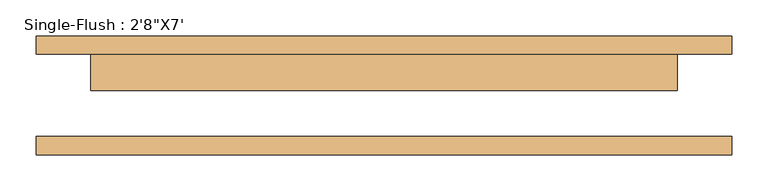
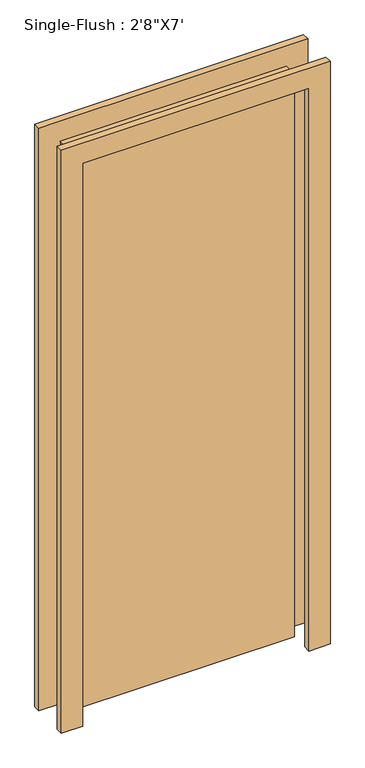
"""IFC4 building model written with IfcOpenShell, lengths in millimetres: door geometry."""

from ifc_helpers import new_model, si_unit, frame, origin, origin_with_axes, place, context, project, spatial, polyline, outline, extrude, source, transform, mapped, element, save


def door_d141acb4(model_context):
    return source(origin(), model_context, "Body", "SweptSolid", [
        extrude(outline(polyline([(2209.8, -482.6), (0.0, -482.6), (0.0, -406.4), (2133.6, -406.4), (2133.6, 406.4), (0.0, 406.4), (0.0, 482.6), (2209.8, 482.6), (2209.8, -482.6)])), frame((0.0, 57.15, 0.0), z_axis=(0.0, 1.0, 0.0), x_axis=(0.0, 0.0, 1.0)), (0.0, 0.0, 1.0), 25.4),
        extrude(outline(polyline([(2209.8, 482.6), (2209.8, -482.6), (0.0, -482.6), (0.0, -406.4), (2133.6, -406.4), (2133.6, 406.4), (0.0, 406.4), (0.0, 482.6), (2209.8, 482.6)])), frame((0.0, -82.55, 0.0), z_axis=(0.0, 1.0, 0.0), x_axis=(0.0, 0.0, 1.0)), (0.0, 0.0, 1.0), 25.4),
        extrude(outline(polyline([(406.4, 6.35), (-406.4, 6.35), (-406.4, 57.15), (406.4, 57.15), (406.4, 6.35)])), origin_with_axes(), (0.0, 0.0, 1.0), 2133.6),
    ])


if __name__ == "__main__":
    model = new_model("IFC4")
    model_context = context("Model", 3, world=origin())
    ifc_project = project(units=[si_unit("LENGTHUNIT", "METRE", prefix="MILLI")], contexts=[model_context])
    site = spatial("IfcSite", under=ifc_project)
    building = spatial("IfcBuilding", under=site)
    placement = place(None, origin())
    door_shape = door_d141acb4(model_context)
    element("IfcDoor", 1, ObjectType="Single-Flush : 2'8\"X7'", at=placement, inside=building, context=model_context, shape_type="MappedRepresentation", body=[
        mapped(door_shape, transform((0.0, 0.0, 0.0), x_axis=(1.0, 0.0, 0.0), y_axis=(0.0, 1.0, 0.0), z_axis=(0.0, 0.0, 1.0))),
    ])
    save(model, "model.ifc")

# Revit data of these elements
# Type "Single-Flush : 2'8\"X7'"
#   Type Mark = "12"
#   Construction Type Id = "MDOOR"
#   Assembly Code = "C1020"
#   Analytic Construction = "Metal"
#   Thickness = 0' - 2"
#   Heat Transfer Coefficient (U) = 0.651978 BTU/(h·ft²·°F)
#   Height = 7' - 0"
#   Trim Projection Ext = 0' - 1"
#   Trim Projection Int = 0' - 1"
#   Trim Width = 0' - 3"
#   Width = 2' - 8"
#   Define Thermal Properties by = 1
#   Door Material = Door - Panel
#   Frame Material = Door - Frame
#   Visual Light Transmittance = 0
#   Solar Heat Gain Coefficient = 0
#   Function = (empty or 0)
#   Wall Closure = (empty or 0)
# Element 1 (IfcDoor, "Single-Flush : 2'8\"X7'")
#   Materials on its faces: "Door - Frame", "Door - Panel"
# Materials
#   "Door - Panel": class "Wood", colour RGB 210 159 95, transparency 0, Cost = 0
#   "Door - Frame": colour RGB 118 70 51, transparency 0, Cost = 0
